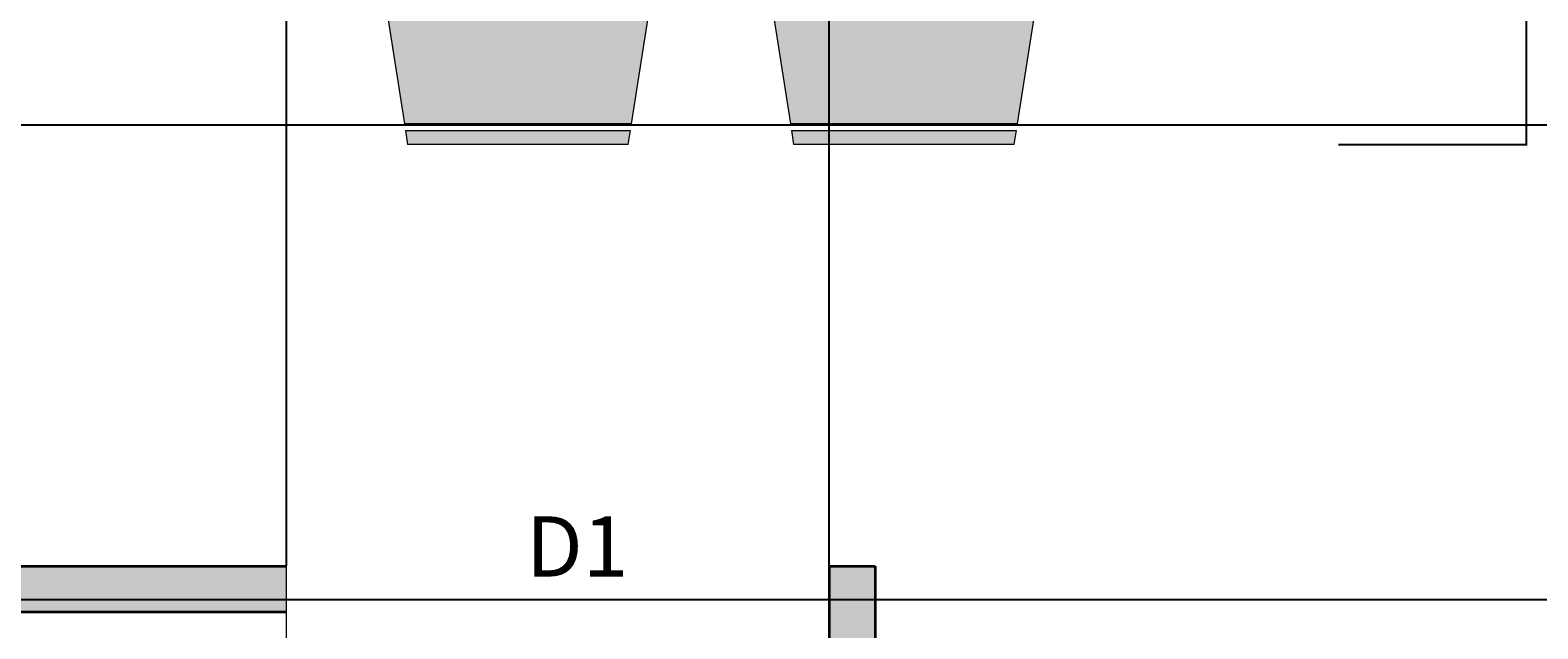
# Model space of a CAD drawing. Units: inches. Extents: x 192 to 1361, y -1362 to 367.
# Tile 15 of 23: x 487 to 783, y -454 to -337. Entities that reach past the tile are written whole.
import ezdxf

# ---------------------------------------------------------------- set-up
doc = ezdxf.new("R2010")
doc.units = ezdxf.units.IN
doc.header["$MEASUREMENT"] = 0
for name, color, linetype, lineweight in [('A-ANNO-DIMS', 2, 'Continuous', 18), ('A-DOOR', 4, 'Continuous', 18), ('A-WALL-PATT', 250, 'Continuous', 13), ('furniture', 32, 'Continuous', 18), ('text', 7, 'Continuous', 18), ('walls', 7, 'Continuous', 35)]:
    doc.layers.add(name, color=color, linetype=linetype, lineweight=lineweight)
doc.layers.add('A-FURN-PATT', color=254, linetype='Continuous', lineweight=13, true_color=0xfeeab9)
doc.styles.get("Standard").update_dxf_attribs({"font": 'arial.ttf'})
doc.dimstyles.get("Standard").update_dxf_attribs({"dimtxt": 0.18, "dimasz": 0.18, "dimexe": 0.18, "dimexo": 0.0625, "dimgap": 0.09, "dimtad": 0, "dimtih": 1, "dimtoh": 1, "dimzin": 0, "dimdsep": 46, "dimlunit": 3, "dimtxsty": 'Standard', "dimcen": 0.09, "dimadec": 0, "dimazin": 0, "dimtfac": 1, "dimtofl": 0, "dimtmove": 0, "dimatfit": 3, "dimfxl": 1, "dimtolj": 1, "dimtzin": 0, "dimarcsym": 0})

# ---------------------------------------------------------------- blocks, each defined once
blk = doc.blocks.new('*U2')
for p, q in [((0, 0), (0, -6)), ((40, 0), (40, -6))]:
    blk.add_line(p, q)
blk.add_lwpolyline([(0, 0), (0, 40), (1.75, 40), (1.75, 0)], close=True)
blk.add_arc((0, 0), 40, 0, 90)
blk = doc.blocks.new('Dining Set - 36 x 72 in.')
for p, q in [((-22, 27.5), (-22.1562, 26.50042)), ((-22, 27.5), (-6, 27.5)), ((-5.8437, 26.49966), (-6, 27.5)), ((6, 27.5), (5.8438, 26.50042)), ((6, 27.5), (22, 27.5)), ((22.1563, 26.49966), (22, 27.5)), ((-5.8416, 26.5), (-22.1534, 26.5)), ((22.1584, 26.5), (5.8466, 26.5)), ((-22.2343, 26.00059), (-23.4847, 17.99762)), ((-22.2304, 26), (-5.7608, 26)), ((-4.5152, 17.99762), (-5.7655, 25.99926)), ((5.7657, 26.00059), (4.5153, 17.99762)), ((5.7696, 26), (22.2392, 26)), ((23.4848, 17.99762), (22.2345, 25.99926)), ((36, 18), (-36, 18)), ((-36, 18), (-36, -18)), ((36, -18), (36, 18)), ((-44.0006, 8.23428), (-35.9976, 9.48474)), ((44.0006, 8.23428), (35.9976, 9.48474)), ((-45.5, 8), (-44.5004, 8.15617)), ((-45.5, 8), (-45.5, -8)), ((-44.5, -8.15843), (-44.5, 8.15338)), ((-44, 8.23041), (-44, -8.23915)), ((44, 8.23041), (44, -8.23915)), ((44.5, -8.15843), (44.5, 8.15338)), ((45.5, 8), (44.5005, 8.15617)), ((45.5, 8), (45.5, -8)), ((-44.4997, -8.15631), (-45.5, -8)), ((-35.9976, -9.48476), (-43.9993, -8.2345)), ((35.9976, -9.48476), (43.9993, -8.2345)), ((44.4997, -8.15631), (45.5, -8)), ((-36, -18), (36, -18)), ((-22.2343, -26.0006), (-23.4847, -17.99762)), ((-4.5152, -17.99762), (-5.7655, -25.99928)), ((5.7657, -26.0006), (4.5153, -17.99762)), ((23.4848, -17.99762), (22.2345, -25.99928)), ((-22.2304, -26), (-5.7608, -26)), ((5.7696, -26), (22.2392, -26)), ((-22, -27.5), (-22.1562, -26.50044)), ((-5.8416, -26.5), (-22.1534, -26.5)), ((-5.8437, -26.49967), (-6, -27.5)), ((6, -27.5), (5.8438, -26.50044)), ((22.1584, -26.5), (5.8466, -26.5)), ((22.1563, -26.49967), (22, -27.5)), ((-22, -27.5), (-6, -27.5)), ((6, -27.5), (22, -27.5))]:
    blk.add_line(p, q)
for points in [[(-36, 15), (-31.1772, 14.97754), (-26.8079, 14.91406), (-22.8538, 14.81543), (-19.276, 14.6875), (-16.0362, 14.53613), (-13.0957, 14.36718), (-10.4159, 14.18652), (-7.9583, 14), (-5.6904, 13.81315), (-3.6035, 13.63021), (-1.6954, 13.45508), (0.0365, 13.29166), (1.5945, 13.14388), (2.9811, 13.01562), (4.1988, 12.9108), (5.25, 12.83333), (6.1393, 12.78613), (6.8802, 12.76823), (7.4883, 12.77767), (7.9792, 12.8125), (8.3685, 12.87077), (8.6719, 12.95052), (8.9049, 13.0498), (9.0833, 13.16666), (9.2205, 13.29899), (9.3216, 13.44401), (9.3895, 13.59879), (9.4271, 13.76041), (9.4373, 13.92594), (9.4232, 14.09245), (9.3875, 14.257), (9.3333, 14.41666), (9.2638, 14.56917), (9.1836, 14.71484), (9.0975, 14.85465), (9.0104, 14.98958), (8.9272, 15.1206), (8.8529, 15.2487), (8.7922, 15.37483), (8.75, 15.5), (8.7305, 15.62467), (8.7344, 15.74739), (8.7617, 15.86621), (8.8125, 15.97916), (8.8867, 16.08431), (8.9844, 16.17968), (9.1055, 16.26334), (9.25, 16.33333), (9.4189, 16.38802), (9.6172, 16.42708), (9.8506, 16.45052), (10.125, 16.45833), (10.4463, 16.45052), (10.8203, 16.42708), (11.2529, 16.38802), (11.75, 16.33333), (12.3184, 16.26318), (12.9694, 16.17838), (13.7151, 16.07991), (14.5677, 15.96875), (15.5395, 15.84586), (16.6426, 15.71224), (17.8893, 15.56884), (19.2917, 15.41666), (20.859, 15.25667), (22.5879, 15.08984), (24.4721, 14.91715), (26.5052, 14.73958), (28.6809, 14.5581), (30.9929, 14.3737), (33.4347, 14.18733), (36, 14)], [(-36, 10), (-28.9766, 10.14274), (-23.1725, 10.20442), (-18.4241, 10.19775), (-14.5677, 10.13541), (-11.4399, 10.03011), (-8.877, 9.89453), (-6.7154, 9.74137), (-4.7917, 9.58333), (-2.9698, 9.43082), (-1.2246, 9.28515), (0.4415, 9.14534), (2.026, 9.01041), (3.5266, 8.87939), (4.9408, 8.7513), (6.266, 8.62516), (7.5, 8.5), (8.6411, 8.37549), (9.6914, 8.2539), (10.6538, 8.13818), (11.5312, 8.03125), (12.3267, 7.93603), (13.043, 7.85547), (13.6831, 7.79248), (14.25, 7.75), (14.7471, 7.7303), (15.1797, 7.73307), (15.5537, 7.75732), (15.875, 7.80208), (16.1494, 7.86637), (16.3828, 7.94922), (16.5811, 8.04964), (16.75, 8.16666), (16.8944, 8.29915), (17.0143, 8.44531), (17.1089, 8.60319), (17.1771, 8.77083), (17.218, 8.94629), (17.2305, 9.1276), (17.2137, 9.31282), (17.1667, 9.5), (17.0895, 9.6875), (16.987, 9.875), (16.8649, 10.0625), (16.7292, 10.25), (16.5856, 10.4375), (16.4401, 10.625), (16.2985, 10.8125), (16.1667, 11), (16.05, 11.18733), (15.9518, 11.3737), (15.8752, 11.5581), (15.8229, 11.73958), (15.798, 11.91715), (15.8034, 12.08984), (15.842, 12.25667), (15.9167, 12.41666), (16.0295, 12.56836), (16.1784, 12.70833), (16.3605, 12.83268), (16.5729, 12.9375), (16.8127, 13.01888), (17.0768, 13.07291), (17.3625, 13.0957), (17.6667, 13.08333), (17.9894, 13.03312), (18.3418, 12.94726), (18.7382, 12.82918), (19.1927, 12.68229), (19.7195, 12.51001), (20.3327, 12.31575), (21.0465, 12.10294), (21.875, 11.875), (22.8357, 11.63354), (23.959, 11.37304), (25.2786, 11.08618), (26.8282, 10.76562), (28.6414, 10.40405), (30.752, 9.99414), (33.1936, 9.52856), (36, 9)], [(-36, 5.5), (-30.7157, 5.3348), (-26.069, 5.20963), (-21.9946, 5.11767), (-18.4271, 5.05208), (-15.3009, 5.00602), (-12.5508, 4.97265), (-10.1112, 4.94515), (-7.9167, 4.91666), (-5.909, 4.88167), (-4.0586, 4.83984), (-2.3429, 4.79215), (-0.7396, 4.73958), (0.7739, 4.6831), (2.22, 4.6237), (3.6213, 4.56233), (5, 4.5), (6.373, 4.43782), (7.7344, 4.3776), (9.0723, 4.32129), (10.375, 4.27083), (11.6309, 4.22819), (12.8281, 4.19531), (13.9551, 4.17415), (15, 4.16666), (15.954, 4.17448), (16.819, 4.19791), (17.6001, 4.23698), (18.3021, 4.29166), (18.9299, 4.36198), (19.4883, 4.44791), (19.9823, 4.54948), (20.4167, 4.66666), (20.7969, 4.79899), (21.1302, 4.94401), (21.4245, 5.09879), (21.6875, 5.26041), (21.9271, 5.42594), (22.1511, 5.59245), (22.3672, 5.757), (22.5834, 5.91666), (22.8065, 6.06868), (23.0404, 6.21093), (23.2879, 6.34147), (23.5521, 6.45833), (23.8358, 6.55957), (24.142, 6.64323), (24.4735, 6.70735), (24.8334, 6.75), (25.2235, 6.76969), (25.642, 6.76692), (26.0858, 6.74267), (26.5521, 6.69791), (27.0379, 6.63362), (27.5404, 6.55078), (28.0565, 6.45036), (28.5834, 6.33333), (29.1242, 6.19987), (29.7071, 6.04687), (30.3661, 5.87044), (31.1354, 5.66666), (32.0493, 5.43164), (33.142, 5.16146), (34.4475, 4.85221), (36, 4.5)], [(-36, -1), (-30.7915, -0.6591), (-26.0195, -0.38216), (-21.6519, -0.16284), (-17.6563, 0.00521), (-14.0005, 0.12833), (-10.6523, 0.21289), (-7.5796, 0.26522), (-4.75, 0.29166), (-2.134, 0.29793), (0.2878, 0.28711), (2.5317, 0.26163), (4.6146, 0.22396), (6.5529, 0.17651), (8.3633, 0.12174), (10.0623, 0.06209), (11.6667, 0), (13.1899, -0.06201), (14.6341, -0.1211), (15.9982, -0.17432), (17.2813, -0.21875), (18.4823, -0.25147), (19.6003, -0.26953), (20.6343, -0.27002), (21.5834, -0.25), (22.4481, -0.20768), (23.2357, -0.14584), (23.9549, -0.06836), (24.6146, 0.02083), (25.2235, 0.11784), (25.7904, 0.21875), (26.3241, 0.31966), (26.8334, 0.41666), (27.3265, 0.50618), (27.8099, 0.58593), (28.2894, 0.65397), (28.7709, 0.70833), (29.2601, 0.74707), (29.763, 0.76823), (30.2855, 0.76985), (30.8334, 0.75), (31.4088, 0.70784), (31.9994, 0.64713), (32.589, 0.57275), (33.1615, 0.48958), (33.7008, 0.4025), (34.1908, 0.3164), (34.6153, 0.23616), (34.9584, 0.16666), (35.2099, 0.11165), (35.3848, 0.07031), (35.504, 0.04069), (35.5886, 0.02083), (35.6594, 0.00879), (35.7377, 0.0026), (35.8442, 0.00032), (36, 0)], [(-36, -6.5), (-27.1843, -6.31267), (-20.084, -6.1263), (-14.469, -5.9419), (-10.1094, -5.76042), (-6.7752, -5.58285), (-4.2363, -5.41016), (-2.2629, -5.24333), (-0.625, -5.08334), (0.8708, -4.93099), (2.2715, -4.78646), (3.5872, -4.64974), (4.8281, -4.52084), (6.0046, -4.39974), (7.127, -4.28646), (8.2053, -4.18099), (9.25, -4.08334), (10.2705, -3.99382), (11.2734, -3.91407), (12.2647, -3.84603), (13.25, -3.79167), (14.2354, -3.75293), (15.2266, -3.73177), (16.2295, -3.73015), (17.25, -3.75), (18.2912, -3.79248), (19.3451, -3.85547), (20.4009, -3.93604), (21.4479, -4.03125), (22.4754, -4.13819), (23.4727, -4.25391), (24.4289, -4.37549), (25.3334, -4.5), (26.1785, -4.62492), (26.9694, -4.74935), (27.7145, -4.87281), (28.4219, -4.99479), (29.1, -5.11483), (29.7572, -5.23242), (30.4016, -5.34709), (31.0417, -5.45834), (31.6837, -5.56437), (32.3262, -5.65821), (32.9658, -5.73153), (33.599, -5.77604), (34.2224, -5.78345), (34.8327, -5.74545), (35.4264, -5.65373), (36, -5.5)], [(-36, -10), (-26.4022, -9.81299), (-18.4675, -9.62891), (-11.9839, -9.45069), (-6.7396, -9.28125), (-2.5226, -9.12354), (0.8789, -8.98047), (3.6769, -8.85498), (6.0833, -8.75), (8.2767, -8.66765), (10.3021, -8.60677), (12.1712, -8.56543), (13.8958, -8.54167), (15.4876, -8.53353), (16.9583, -8.53907), (18.3197, -8.55632), (19.5834, -8.58334), (20.7616, -8.61841), (21.8685, -8.66081), (22.9188, -8.71004), (23.9271, -8.76563), (24.9081, -8.82707), (25.8763, -8.89388), (26.8465, -8.96558), (27.8334, -9.04167), (28.8474, -9.12118), (29.8828, -9.20117), (30.93, -9.27824), (31.9792, -9.34896), (33.0205, -9.40991), (34.0443, -9.45768), (35.0407, -9.48885), (36, -9.5)], [(-36, -14.5), (-30.0881, -14.33513), (-25.0332, -14.21224), (-20.7312, -14.12647), (-17.0781, -14.07292), (-13.97, -14.04671), (-11.3027, -14.04297), (-8.9724, -14.05681), (-6.875, -14.08334), (-4.9224, -14.11833), (-3.0905, -14.16016), (-1.3709, -14.20785), (0.2448, -14.26042), (1.7647, -14.3169), (3.1973, -14.3763), (4.5507, -14.43767), (5.8333, -14.5), (7.0554, -14.5621), (8.235, -14.62175), (9.3922, -14.67652), (10.5469, -14.72396), (11.7192, -14.76164), (12.929, -14.78711), (14.1965, -14.79794), (15.5417, -14.79167), (16.9933, -14.76424), (18.6152, -14.70508), (20.4804, -14.60197), (22.6615, -14.44271), (25.2312, -14.21509), (28.2624, -13.9069), (31.8277, -13.50594), (36, -13)]]:
    blk.add_lwpolyline(points)
blk = doc.blocks.new('dining area')
at = {"layer": 'furniture', "xscale": 0.6659924291999282, "yscale": 0.6659924291999282, "zscale": 0.6659924291999282, "rotation": 90}
blk.add_blockref('Dining Set - 36 x 72 in.', (-0.439, 20.507), dxfattribs=at)
blk = doc.blocks.new('*D44')
at = {"layer": 'A-ANNO-DIMS', "color": 0, "lineweight": -2, "transparency": 16777216}
for p, q in [((743.7, -210.74), (780.69, -210.74)), ((780.51, -210.92), (780.51, -284.83)), ((780.51, -359.11), (780.51, -285.2)), ((743.7, -359.29), (780.69, -359.29))]:
    blk.add_line(p, q, dxfattribs=at)
at = {"layer": 'A-ANNO-DIMS', "color": 0, "transparency": 16777216}
for points in [[(780.48, -210.92), (780.54, -210.92), (780.51, -210.74)], [(780.48, -359.11), (780.54, -359.11), (780.51, -359.29)]]:
    blk.add_solid(points, dxfattribs=at)
at = {"layer": 'Defpoints', "color": 0, "transparency": 16777216}
for p in [(743.64, -210.74), (780.51, -210.74), (743.64, -359.29)]:
    blk.add_point(p, dxfattribs=at)
at = {"layer": 'A-ANNO-DIMS', "color": 0, "transparency": 16777216, "insert": (780.51, -285.01), "char_height": 0.18, "attachment_point": 5}
blk.add_mtext('\\A1;149', dxfattribs=at)
blk = doc.blocks.new('*D70')
at = {"layer": 'A-ANNO-DIMS', "color": 0, "lineweight": -2, "transparency": 16777216}
for p, q in [((537.57, -441.84), (537.57, 367.39)), ((537.75, 367.21), (590.28, 367.21)), ((643.71, 367.21), (591.19, 367.21)), ((643.89, -441.84), (643.89, 367.39))]:
    blk.add_line(p, q, dxfattribs=at)
at = {"layer": 'A-ANNO-DIMS', "color": 0, "transparency": 16777216}
for points in [[(537.75, 367.24), (537.75, 367.18), (537.57, 367.21)], [(643.71, 367.24), (643.71, 367.18), (643.89, 367.21)]]:
    blk.add_solid(points, dxfattribs=at)
at = {"layer": 'Defpoints', "color": 0, "transparency": 16777216}
for p in [(643.89, 367.21), (537.57, -441.9), (643.89, -441.9)]:
    blk.add_point(p, dxfattribs=at)
at = {"layer": 'A-ANNO-DIMS', "color": 0, "transparency": 16777216, "insert": (590.73, 367.21), "char_height": 0.18, "attachment_point": 5}
blk.add_mtext('\\A1;106.32', dxfattribs=at)
blk = doc.blocks.new('*D71')
at = {"layer": 'A-ANNO-DIMS', "color": 0, "lineweight": -2, "transparency": 16777216}
for p, q in [((784.74, -355.5), (192.16, -355.5)), ((192.34, -355.68), (192.34, -401.82)), ((192.34, -448.32), (192.34, -402.18)), ((784.74, -448.5), (192.16, -448.5))]:
    blk.add_line(p, q, dxfattribs=at)
at = {"layer": 'A-ANNO-DIMS', "color": 0, "transparency": 16777216}
for points in [[(192.31, -355.68), (192.37, -355.68), (192.34, -355.5)], [(192.31, -448.32), (192.37, -448.32), (192.34, -448.5)]]:
    blk.add_solid(points, dxfattribs=at)
at = {"layer": 'Defpoints', "color": 0, "transparency": 16777216}
for p in [(784.8, -355.5), (192.34, -448.5), (784.8, -448.5)]:
    blk.add_point(p, dxfattribs=at)
at = {"layer": 'A-ANNO-DIMS', "color": 0, "transparency": 16777216, "insert": (192.34, -402), "char_height": 0.18, "attachment_point": 5}
blk.add_mtext('\\A1;93', dxfattribs=at)

msp = doc.modelspace()

# ---------------------------------------------------------------- hatches: boundary and pattern name
at = {"layer": 'A-FURN-PATT'}
h = msp.add_hatch(color=256, dxfattribs=at)
h.dxf.hatch_style = 1
h.paths.add_polyline_path([(605.1742, -214.7906), (560.6934, -214.7906), (557.3171, -236.398), (608.5502, -236.398)])
h.paths.add_polyline_path([(604.5412, -210.7392), (561.3264, -210.7392), (560.9044, -213.4402), (604.9632, -213.4402)])
h.paths.add_polyline_path([(680.8, -214.7906), (636.3191, -214.7906), (632.9429, -236.398), (684.176, -236.398)])
h.paths.add_polyline_path([(680.1669, -210.7392), (636.9522, -210.7392), (636.5302, -213.4402), (680.589, -213.4402)])
h.paths.add_polyline_path([(523.5135, -259.398), (501.9062, -262.7741), (501.9062, -307.2549), (523.5135, -310.6311)])
h.paths.add_polyline_path([(500.5557, -262.9851), (497.8548, -263.4072), (497.8548, -306.6219), (500.5557, -307.0439)])
h.paths.add_polyline_path([(608.5502, -333.6311), (557.3171, -333.6311), (560.6934, -355.2385), (605.1742, -355.2385)])
h.paths.add_polyline_path([(604.9632, -356.5889), (560.9044, -356.5889), (561.3264, -359.2899), (604.5412, -359.2899)])
h.paths.add_polyline_path([(680.589, -356.5889), (636.5302, -356.5889), (636.9522, -359.2899), (680.1669, -359.2899)])
h.paths.add_polyline_path([(684.176, -333.6311), (632.9429, -333.6311), (636.3191, -355.2385), (680.8, -355.2385)])
h.paths.add_polyline_path([(739.5872, -262.7741), (717.9798, -259.398), (717.9798, -310.6311), (739.5872, -307.2549)])
h.paths.add_polyline_path([(743.6386, -263.4072), (740.9376, -262.9851), (740.9376, -307.0439), (743.6386, -306.6219)])
at = {"layer": 'A-WALL-PATT'}
h = msp.add_hatch(color=256, dxfattribs=at)
h.dxf.hatch_style = 1
h.paths.add_polyline_path([(309.5452, 191.102), (300.5452, 191.102), (300.5452, -126.898), (309.5452, -126.898), (309.5452, -117.898)])
h.paths.add_polyline_path([(420.798, 191.102), (337.3229, 191.102), (337.3229, 182.102), (420.798, 182.102)])
h.paths.add_polyline_path([(518.5452, 182.102), (625.4022, 182.102), (625.4022, 191.102), (509.5452, 191.102), (509.5452, 114.3262), (518.5452, 114.3262)])
h.paths.add_polyline_path([(842.5452, 191.102), (763.4438, 191.102), (763.4438, 182.102), (833.5452, 182.102), (833.5452, 161.1615), (836.8088, 161.1615), (842.5452, 161.1615)])
h.paths.add_polyline_path([(842.5452, -16.5675), (833.5452, -16.5675), (833.5452, -60.4996), (784.8041, -60.4996), (784.8041, -354.6796), (793.8041, -354.6796), (793.8041, -69.4996), (1094.1252, -69.4996), (1094.1252, -60.4996), (842.5452, -60.4996)])
h.paths.add_polyline_path([(518.5452, 36.602), (509.5452, 36.602), (509.5452, -117.898), (420.2204, -117.898), (420.2204, -126.898), (518.5452, -126.898)])
h.paths.add_polyline_path([(474.8041, -377.0384), (465.8041, -377.0384), (465.8041, -381.5384), (465.8041, -450.898), (537.5717, -450.898), (537.5717, -441.898), (474.8041, -441.898)])
h.paths.add_polyline_path([(1162.8041, -380.6763), (1204.3001, -380.6763), (1204.3001, -375.6763), (1195.1471, -375.6763), (1153.8041, -375.6763), (1153.8041, -448.4996), (856.5691, -448.4996), (856.5691, -457.4996), (1162.8041, -457.4996)])
h.paths.add_polyline_path([(1162.8041, -525.128), (1153.8041, -525.128), (1153.8041, -597.4996), (1162.8041, -597.4996)], flags=17)
h.paths.add_polyline_path([(1162.8041, -60.4996), (1153.8041, -60.4996), (1153.8041, -69.4996), (1153.8041, -177.4733), (1205.8889, -177.4733), (1205.8889, -172.4733), (1162.8041, -172.4733)])
h.paths.add_polyline_path([(980.5799, -525.686), (971.5799, -525.686), (971.5799, -597.4996), (980.5799, -597.4996)], flags=17)
h.paths.add_polyline_path([(856.5691, -448.4996), (798.7542, -448.4996), (784.8041, -448.4996), (784.8041, -457.4996), (847.5691, -457.4996), (847.5691, -597.4996), (784.8041, -597.4996), (784.8041, -606.4996), (1273.5658, -606.4996), (1273.5658, -597.4996), (856.5691, -597.4996)])
h.paths.add_polyline_path([(1273.5658, -773.892), (1099.8366, -773.892), (1099.8366, -851.9362), (1108.8366, -851.9362), (1108.8366, -782.892), (1273.5658, -782.892)])
h.paths.add_polyline_path([(1108.8366, -982.9214), (1099.8366, -982.9214), (1099.8366, -1067.6246), (1037.7563, -1067.6246), (1037.7563, -1076.6246), (1108.8366, -1076.6246)])
h.paths.add_polyline_path([(835.078, -1067.6246), (758.8458, -1067.6246), (758.8458, -940.2324), (749.8458, -940.2324), (749.8458, -963.172), (749.8458, -970.4644), (749.8458, -1076.6246), (835.078, -1076.6246)])
h.paths.add_polyline_path([(450.307, -1066.9838), (441.307, -1066.9838), (441.307, -1076.6246), (450.307, -1076.6246)])
h.paths.add_polyline_path([(492.8925, -756.4415), (274.8925, -756.4415), (274.8925, -765.4415), (492.8925, -765.4415)])
h.paths.add_polyline_path([(283.8925, -835.2244), (274.8925, -835.2244), (274.8925, -914.4415), (492.8925, -914.4415), (492.8925, -839.9415), (483.8925, -839.9415), (483.8925, -905.4415), (283.8925, -905.4415)])
h.paths.add_polyline_path([(283.8925, -441.898), (283.8925, -375.4296), (281.6021, -375.4296), (281.6021, -399.4121), (274.8925, -399.4121), (274.8925, -441.898), (274.8925, -684.5089), (283.8925, -684.5089)])
h = msp.add_hatch(color=256, dxfattribs=at)
h.dxf.hatch_style = 1
h.paths.add_polyline_path([(652.8925, -441.898), (643.8925, -441.898), (643.8925, -457.8461), (643.8925, -564.167), (643.8925, -905.4415), (578.0245, -905.4415), (578.0245, -914.4415), (643.8925, -914.4415), (643.8925, -969.5484), (652.6138, -969.5484), (652.6138, -963.172), (652.6138, -914.556)])
h.paths.add_polyline_path([(509.5452, 191.102), (504.3983, 191.102), (504.3983, 182.102), (509.5452, 182.102)])

# ---------------------------------------------------------------- linework, layer by layer
at = {"layer": 'walls'}
for p, q in [((474.8041, -441.898), (537.5717, -441.898)), ((643.8925, -441.898), (643.8925, -905.4415)), ((643.8925, -441.898), (652.8925, -441.898)), ((652.8925, -441.898), (652.8925, -969.5484)), ((465.8041, -450.898), (537.5717, -450.898))]:
    msp.add_line(p, q, dxfattribs=at)

# ---------------------------------------------------------------- block references
at = {"layer": 'A-DOOR', "xscale": 2.658020973626523, "yscale": 2.658020973626523, "zscale": 2.658020973626523, "rotation": 180}
msp.add_blockref('*U2', (643.8925, -457.8461), dxfattribs=at)
at = {"layer": 'furniture', "xscale": 4.055482377011951, "yscale": 4.055482377011951, "zscale": 4.055482377011951, "rotation": 90}
msp.add_blockref('dining area', (703.9121, -283.2344), dxfattribs=at)

# ---------------------------------------------------------------- texts
at = {"layer": 'text'}
msp.add_text('D1', height=11.81288, dxfattribs=at).set_placement((584.5455, -443.9657))

# ---------------------------------------------------------------- dimensions: what is measured, and where the dimension line sits
at = {"layer": 'A-ANNO-DIMS'}
dim = msp.add_linear_dim(base=(643.8925, 367.2097), p1=(537.5717, -441.898), p2=(643.8925, -441.898), dimstyle='Standard', override={"dimdec": 2, "dimlfac": 1, "dimrnd": 0, "dimzin": 0, "dimdsep": 46, "dimlunit": 2}, dxfattribs=at)
dim.commit()
dim.dimension.update_dxf_attribs({"geometry": '*D70', "text_midpoint": (590.7321, 367.2097)})
for base, p1, p2, picture, middle in [((780.5061, -210.7392), (743.6386, -359.2899), (743.6386, -210.7392), '*D44', (780.5061, -285.0145)), ((192.3425, -448.4996), (784.8041, -355.4994), (784.8041, -448.4996), '*D71', (192.3425, -401.9995))]:
    dim = msp.add_linear_dim(base=base, p1=p1, p2=p2, angle=90, dimstyle='Standard', override={"dimdec": 0, "dimlfac": 1, "dimrnd": 0, "dimzin": 0, "dimdsep": 46, "dimlunit": 2}, dxfattribs=at)
    dim.commit()
    dim.dimension.update_dxf_attribs({"geometry": picture, "text_midpoint": middle})

doc.saveas('drawing.dxf')
